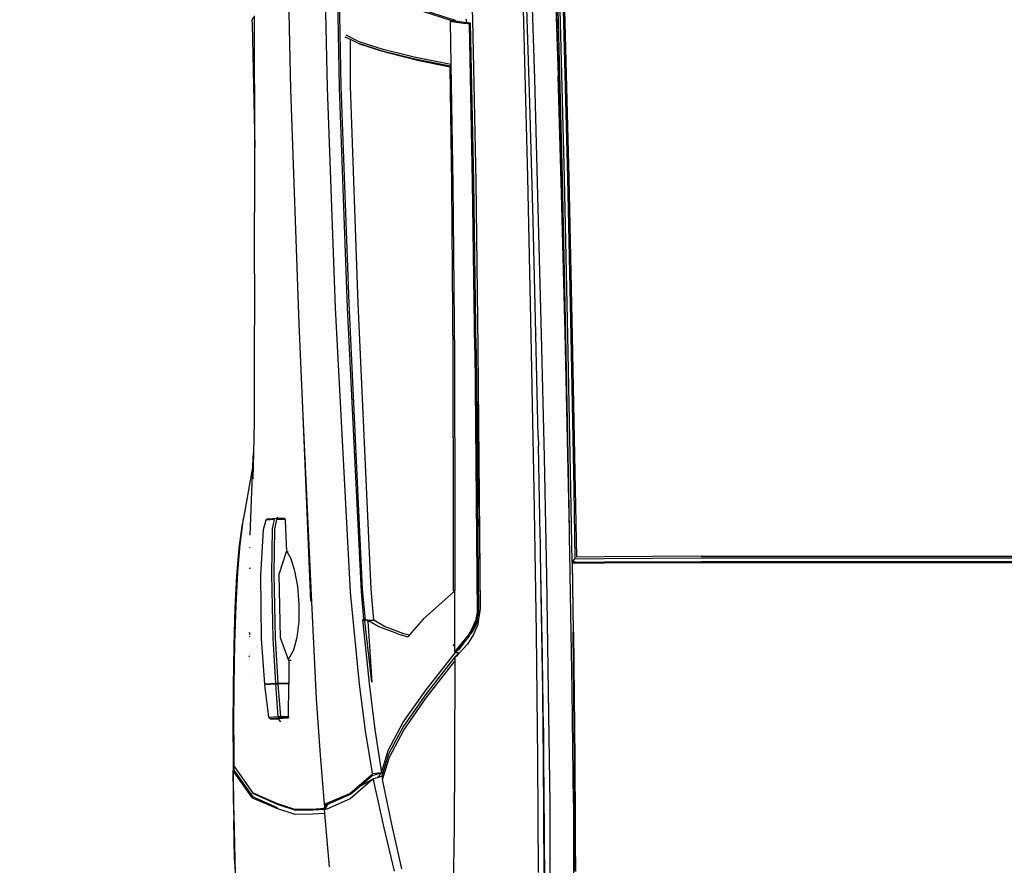
# Model space of a CAD drawing. Units: inches. Extents: x 1319 to 2030, y 219 to 1069.
# Tile 9 of 28: x 1417 to 1461, y 392 to 430. Entities that reach past the tile are written whole.
import ezdxf

# ---------------------------------------------------------------- set-up
doc = ezdxf.new("R2010")
doc.units = ezdxf.units.IN
doc.header["$MEASUREMENT"] = 0
doc.layers.get('0').update_dxf_attribs({"color": 12})
doc.layers.add('A-ANNO-DIMS', color=2, linetype='Continuous', lineweight=18)
doc.layers.add('C-PRKG-VEHC', color=8, linetype='Continuous', lineweight=13)
doc.layers.add('Edges', color=250, linetype='Continuous')
doc.styles.get("Standard").update_dxf_attribs({"font": 'arial.ttf'})
doc.dimstyles.get("Standard").update_dxf_attribs({"dimtxt": 7, "dimasz": 0.18, "dimexe": 0.18, "dimexo": 0.0625, "dimgap": 0.09, "dimtad": 0, "dimtih": 1, "dimtoh": 1, "dimzin": 0, "dimdsep": 46, "dimlunit": 3, "dimtxsty": 'Standard', "dimcen": 0.09, "dimadec": 0, "dimazin": 0, "dimtfac": 1, "dimtofl": 0, "dimtmove": 0, "dimatfit": 3, "dimfxl": 1, "dimtolj": 1, "dimtzin": 0, "dimarcsym": 0})

# ---------------------------------------------------------------- blocks, each defined once
blk = doc.blocks.new('Nissan Qashqai pl')
at = {"layer": 'Edges'}
for p, q in [((10.4706, 11.5566), (10.4706, 12.2875)), ((10.4726, 11.5567), (10.4726, 12.2875)), ((10.4764, 11.5569), (10.4764, 12.2872)), ((10.4776, 11.5567), (10.4776, 12.2874)), ((10.4706, 11.5566), (10.4711, 11.4469)), ((10.4731, 11.4469), (10.4726, 11.5567)), ((10.4769, 11.4474), (10.4764, 11.5569)), ((10.4781, 11.4469), (10.4776, 11.5567)), ((10.4711, 11.4469), (10.4715, 11.416)), ((10.4735, 11.414), (10.4731, 11.4469)), ((10.4773, 11.4146), (10.4769, 11.4474)), ((10.4785, 11.4111), (10.4781, 11.4469)), ((10.3947, 11.4148), (10.2218, 11.4114)), ((10.4715, 11.416), (10.3947, 11.4148)), ((10.4773, 11.4146), (10.4773, 11.4107)), ((10.7933, 11.4143), (10.827, 11.4145)), ((10.0431, 11.4075), (9.8673, 11.4031)), ((9.8673, 11.4012), (10.043, 11.4055)), ((10.2215, 11.406), (10.0429, 11.4021)), ((10.2216, 11.4037), (10.0429, 11.3998)), ((10.043, 11.4055), (10.2218, 11.4094)), ((10.2218, 11.4114), (10.0431, 11.4075)), ((10.3564, 11.406), (10.2175, 11.4028)), ((10.3945, 11.4094), (10.2215, 11.406)), ((10.3947, 11.4071), (10.2216, 11.4037)), ((10.2218, 11.4094), (10.3947, 11.4128)), ((10.4416, 11.4077), (10.3564, 11.406)), ((10.4773, 11.4107), (10.3945, 11.4094)), ((10.3947, 11.4128), (10.4735, 11.414)), ((10.4416, 11.4078), (10.3947, 11.4071)), ((10.4519, 11.4079), (10.4416, 11.4077)), ((10.4519, 11.4079), (10.4416, 11.4078)), ((10.4416, 11.4077), (10.4416, 11.4078)), ((10.4524, 11.408), (10.4519, 11.4079)), ((10.4519, 11.4079), (10.4519, 11.4079)), ((10.4524, 11.4079), (10.4519, 11.4079)), ((10.4524, 11.4079), (10.4524, 11.408)), ((10.4533, 11.408), (10.4524, 11.408)), ((10.4533, 11.4079), (10.4524, 11.4079)), ((10.4638, 11.4081), (10.4533, 11.4079)), ((10.4638, 11.4081), (10.4533, 11.408)), ((10.4533, 11.4079), (10.4533, 11.408)), ((10.4914, 11.4087), (10.4638, 11.4081)), ((10.4773, 11.4107), (10.4735, 11.414)), ((10.4773, 11.4107), (10.5561, 11.4119)), ((10.4773, 11.4107), (10.4785, 11.4111)), ((10.5563, 11.4123), (10.4785, 11.4111)), ((10.6223, 11.4109), (10.4914, 11.4087)), ((10.6996, 11.4134), (10.5561, 11.4119)), ((10.5563, 11.4123), (10.6999, 11.4138)), ((10.7493, 11.4125), (10.6223, 11.4109)), ((10.7722, 11.4138), (10.6996, 11.4134)), ((10.6999, 11.4138), (10.7722, 11.4142)), ((10.7493, 11.4125), (11.0294, 11.4126)), ((10.7722, 11.4142), (10.7889, 11.4143)), ((10.7722, 11.4142), (10.7722, 11.4138)), ((10.7889, 11.4139), (10.7722, 11.4138)), ((10.7889, 11.4139), (10.7889, 11.4143)), ((10.7889, 11.4143), (10.7923, 11.4143)), ((10.7923, 11.4139), (10.7889, 11.4139)), ((10.7923, 11.4139), (10.7923, 11.4143)), ((10.7923, 11.4143), (10.7933, 11.4143)), ((10.7933, 11.4139), (10.7923, 11.4139)), ((10.7933, 11.4139), (10.7933, 11.4143)), ((10.8267, 11.4141), (10.7933, 11.4139)), ((9.6472, 11.3861), (9.9278, 11.3949)), ((9.8673, 11.4031), (9.701, 11.3983)), ((9.7011, 11.3963), (9.8673, 11.4012)), ((9.8673, 11.3977), (9.7014, 11.3929)), ((9.8673, 11.3954), (9.7014, 11.3906)), ((9.8565, 11.3931), (9.9794, 11.3967)), ((10.0429, 11.4021), (9.8673, 11.3977)), ((10.0429, 11.3998), (9.8673, 11.3954)), ((10.0747, 11.3991), (9.9278, 11.3949)), ((9.9794, 11.3967), (10.0965, 11.3998)), ((10.2043, 11.4025), (10.0747, 11.3991)), ((10.0965, 11.3998), (10.0998, 11.3999)), ((10.0998, 11.3999), (10.2043, 11.4025)), ((10.2175, 11.4028), (10.2043, 11.4025)), ((10.3586, 11.3791), (10.4931, 11.3817)), ((10.4931, 11.3817), (10.6237, 11.3839)), ((10.6237, 11.3839), (10.7502, 11.3855)), ((10.7502, 11.3855), (10.968, 11.3857)), ((9.9312, 11.3681), (10.0776, 11.3722)), ((10.0776, 11.3722), (10.2201, 11.3759)), ((10.2201, 11.3759), (10.3586, 11.3791)), ((10.3353, 11.3725), (10.2203, 11.3699)), ((10.3353, 11.3725), (10.346, 11.3727)), ((10.4477, 11.3747), (10.346, 11.3727)), ((10.5572, 11.3704), (10.3955, 11.368)), ((10.4537, 11.3749), (10.4477, 11.3747)), ((10.4537, 11.3749), (10.4538, 11.3749)), ((10.4681, 11.3752), (10.4538, 11.3749)), ((10.4676, 11.3751), (10.4538, 11.3749)), ((10.5576, 11.3766), (10.4676, 11.3751)), ((10.5566, 11.3765), (10.4676, 11.3751)), ((10.4676, 11.3751), (10.4676, 11.3751)), ((10.5866, 11.3772), (10.4681, 11.3752)), ((10.5566, 11.3765), (10.7, 11.378)), ((10.7004, 11.372), (10.5572, 11.3704)), ((10.6649, 11.3783), (10.5576, 11.3766)), ((10.6649, 11.3783), (10.5866, 11.3772)), ((10.6908, 11.3785), (10.6649, 11.3783)), ((10.6649, 11.3783), (10.6772, 11.3784)), ((10.6966, 11.3787), (10.6772, 11.3784)), ((10.6772, 11.3784), (10.6908, 11.3785)), ((10.6991, 11.3786), (10.6908, 11.3785)), ((10.7144, 11.3788), (10.6966, 11.3787)), ((10.6999, 11.3786), (10.6991, 11.3786)), ((10.6999, 11.3786), (10.7808, 11.3793)), ((10.7144, 11.3788), (10.6999, 11.3786)), ((10.7, 11.378), (10.8279, 11.3787)), ((10.8279, 11.3727), (10.7004, 11.372)), ((10.7239, 11.3789), (10.7144, 11.3788)), ((10.7248, 11.3789), (10.7239, 11.3789)), ((10.7808, 11.3793), (10.7248, 11.3789)), ((10.7808, 11.3793), (10.8711, 11.3796)), ((9.9583, 11.363), (9.651, 11.3536)), ((9.6514, 11.3592), (9.9312, 11.3681)), ((10.0423, 11.3607), (9.8673, 11.3563)), ((10.091, 11.3666), (9.9583, 11.363)), ((10.2211, 11.3646), (10.0423, 11.3607)), ((10.2191, 11.3699), (10.091, 11.3666)), ((10.2202, 11.3699), (10.2191, 11.3699)), ((10.2202, 11.3699), (10.2203, 11.3699)), ((10.3955, 11.368), (10.2211, 11.3646)), ((9.8673, 11.3563), (9.7029, 11.3516)), ((10.0472, 11.3018), (10.2357, 11.3043)), ((10.2357, 11.3043), (10.53, 11.3068)), ((10.2367, 11.3022), (10.5351, 11.305)), ((10.2369, 11.3008), (10.5348, 11.3036)), ((10.4153, 11.3058), (10.2954, 11.3046)), ((10.4153, 11.3058), (10.4174, 11.3058)), ((10.4174, 11.3058), (10.4181, 11.3058)), ((10.4181, 11.3058), (10.4182, 11.3058)), ((10.4182, 11.3058), (10.53, 11.3068)), ((10.53, 11.3068), (10.5301, 11.3068)), ((10.5301, 11.3068), (10.5323, 11.3065)), ((10.5323, 11.3065), (10.5419, 11.3051)), ((10.5422, 11.3021), (10.5348, 11.3036)), ((10.5424, 11.3035), (10.5351, 11.305)), ((10.5366, 11.3048), (10.536, 11.305)), ((10.5379, 11.3052), (10.5381, 11.305)), ((10.5419, 11.3051), (10.5463, 11.3031)), ((10.5419, 11.3051), (10.5479, 11.3042)), ((10.5472, 11.3014), (10.5424, 11.3035)), ((10.5463, 11.3031), (10.5551, 11.2984)), ((10.5479, 11.3042), (10.5589, 11.2991)), ((9.696, 11.2932), (9.8644, 11.2982)), ((9.8644, 11.2982), (10.0472, 11.3018)), ((9.8678, 11.2935), (9.8677, 11.291)), ((9.8681, 11.2959), (9.8678, 11.2935)), ((10.0476, 11.2996), (9.8681, 11.2959)), ((9.8681, 11.2959), (9.869, 11.2946)), ((9.8689, 11.2927), (9.8686, 11.2879)), ((9.869, 11.2946), (9.8689, 11.2927)), ((10.0477, 11.2982), (9.869, 11.2946)), ((10.2367, 11.3022), (10.0476, 11.2996)), ((10.2369, 11.3008), (10.0477, 11.2982)), ((10.5522, 11.2977), (10.5422, 11.3021)), ((10.5546, 11.2982), (10.5472, 11.3014)), ((10.5598, 11.2935), (10.5522, 11.2977)), ((10.5583, 11.296), (10.5546, 11.2982)), ((10.5551, 11.2984), (10.5583, 11.296)), ((10.5612, 11.2944), (10.5583, 11.296)), ((10.5589, 11.2991), (10.57, 11.2925)), ((10.5764, 11.28), (10.5598, 11.2935)), ((10.5683, 11.2885), (10.5612, 11.2944)), ((10.57, 11.2925), (10.5811, 11.2822)), ((9.8637, 11.291), (9.8643, 11.291)), ((9.8643, 11.291), (9.8677, 11.291)), ((9.8675, 11.2887), (9.8655, 11.2754)), ((9.8686, 11.2879), (9.8665, 11.2747)), ((9.8677, 11.291), (9.8675, 11.2887)), ((10.5683, 11.2885), (10.573, 11.285)), ((10.575, 11.2829), (10.5683, 11.2885)), ((10.573, 11.285), (10.5769, 11.2818)), ((10.5776, 11.2808), (10.575, 11.2829)), ((10.5796, 11.2824), (10.5796, 11.2787)), ((10.5811, 11.2822), (10.5821, 11.2808)), ((10.5811, 11.2822), (10.5834, 11.28)), ((10.5821, 11.2808), (10.5834, 11.2793)), ((9.8652, 11.2788), (9.8516, 11.2363)), ((9.8652, 11.2738), (9.8516, 11.2313)), ((9.8652, 11.2738), (9.8652, 11.2788)), ((9.8655, 11.2754), (9.8652, 11.2738)), ((9.8652, 11.2735), (9.8665, 11.2747)), ((9.8652, 11.2738), (9.8652, 11.2738)), ((9.8652, 11.2738), (9.8652, 11.2735)), ((9.8652, 11.2735), (9.8664, 11.2728)), ((9.8665, 11.2747), (9.8664, 11.2728)), ((9.8664, 11.2728), (9.9149, 11.2736)), ((9.9149, 11.2736), (9.9066, 11.2322)), ((9.9169, 11.2728), (9.9086, 11.2313)), ((9.9177, 11.2728), (9.9106, 11.2373)), ((9.9149, 11.2736), (10.0505, 11.276)), ((9.9177, 11.2728), (9.9169, 11.2728)), ((10.0501, 11.2747), (9.9177, 11.2728)), ((10.2453, 11.2762), (10.0501, 11.2747)), ((10.0505, 11.276), (10.2453, 11.2777)), ((10.2453, 11.2777), (10.4289, 11.2783)), ((10.4292, 11.2767), (10.2453, 11.2762)), ((10.4289, 11.2783), (10.5092, 11.2783)), ((10.5099, 11.2768), (10.4292, 11.2767)), ((10.5099, 11.2768), (10.5092, 11.2783)), ((10.5092, 11.2783), (10.5094, 11.2783)), ((10.5094, 11.2783), (10.51, 11.2776)), ((10.5783, 11.2783), (10.5094, 11.2783)), ((10.51, 11.2776), (10.5099, 11.2768)), ((10.51, 11.2776), (10.5419, 11.2423)), ((10.5705, 11.2771), (10.5709, 11.2767)), ((10.5709, 11.2767), (10.5719, 11.2759)), ((10.5783, 11.2783), (10.5764, 11.28)), ((10.5796, 11.2787), (10.5776, 11.2808)), ((10.5776, 11.2808), (10.5783, 11.2783)), ((10.5796, 11.2787), (10.5783, 11.2783)), ((10.6215, 11.2456), (10.5796, 11.2787)), ((10.5825, 11.2806), (10.5834, 11.2793)), ((10.5834, 11.28), (10.5851, 11.2783)), ((10.5834, 11.2793), (10.5835, 11.2793)), ((10.5835, 11.2793), (10.584, 11.2787)), ((10.584, 11.2789), (10.584, 11.2793)), ((10.584, 11.2787), (10.584, 11.2789)), ((10.584, 11.2787), (10.6261, 11.2458)), ((10.584, 11.2787), (10.5851, 11.2783)), ((10.5843, 11.2787), (10.584, 11.2787)), ((10.5847, 11.2787), (10.5843, 11.2787)), ((10.5851, 11.2783), (10.5892, 11.2783)), ((10.6306, 11.2459), (10.5892, 11.2783)), ((10.5892, 11.2783), (10.6988, 11.2779)), ((10.6988, 11.2779), (10.7769, 11.2774)), ((10.7769, 11.2774), (10.858, 11.2759)), ((9.9106, 11.2373), (9.9018, 11.2021)), ((10.5419, 11.2423), (10.56, 11.2265)), ((10.6583, 11.2197), (10.6215, 11.2456)), ((10.6261, 11.2458), (10.6627, 11.22)), ((10.6671, 11.2203), (10.6306, 11.2459)), ((9.9066, 11.2322), (9.8978, 11.197)), ((9.9086, 11.2313), (9.8998, 11.196)), ((10.56, 11.2265), (10.5584, 11.2206)), ((10.56, 11.2265), (10.5617, 11.2251)), ((10.5584, 11.2206), (10.5502, 11.1986)), ((10.5584, 11.2136), (10.5617, 11.2251)), ((10.69, 11.2028), (10.6583, 11.2197)), ((10.6627, 11.22), (10.6943, 11.2032)), ((10.6976, 11.2041), (10.6671, 11.2203)), ((10.8239, 11.2181), (10.7754, 11.2071)), ((10.5584, 11.2136), (10.5502, 11.1916)), ((10.6943, 11.2032), (10.7155, 11.1969)), ((10.7228, 11.1965), (10.6976, 11.2041)), ((10.7754, 11.2071), (10.7228, 11.1965)), ((10.8264, 11.21), (10.7776, 11.1982)), ((9.8978, 11.197), (9.8891, 11.1701)), ((9.8911, 11.1693), (9.8998, 11.196)), ((9.9018, 11.2021), (9.8931, 11.1752)), ((10.5502, 11.1986), (10.543, 11.1865)), ((10.6664, 11.1875), (10.7155, 11.1952)), ((10.7155, 11.1952), (10.69, 11.2028)), ((10.7155, 11.1957), (10.7155, 11.1969)), ((10.7155, 11.1969), (10.7192, 11.1957)), ((10.7209, 11.1902), (10.7155, 11.1957)), ((10.7155, 11.1952), (10.7155, 11.1957)), ((10.7186, 11.1848), (10.7155, 11.1952)), ((10.7155, 11.1952), (10.7165, 11.1851)), ((10.7192, 11.1957), (10.7228, 11.1965)), ((10.7192, 11.1957), (10.7209, 11.1902)), ((10.7776, 11.1982), (10.7247, 11.1867)), ((10.5079, 11.1835), (10.1849, 11.1687)), ((10.543, 11.1865), (10.5079, 11.1835)), ((10.5502, 11.1916), (10.543, 11.1795)), ((10.543, 11.1795), (10.543, 11.1865)), ((10.5439, 11.1796), (10.613, 11.1841)), ((10.5458, 11.1742), (10.6144, 11.1813)), ((10.613, 11.1841), (10.547, 11.1767)), ((10.6144, 11.1813), (10.6664, 11.1875)), ((10.7137, 11.1846), (10.6678, 11.177)), ((10.7165, 11.1851), (10.7137, 11.1846)), ((10.7177, 11.1838), (10.7165, 11.1851)), ((10.7387, 11.1593), (10.7177, 11.1838)), ((10.7312, 11.1701), (10.7186, 11.1848)), ((10.7209, 11.1902), (10.7221, 11.1861)), ((10.7221, 11.1861), (10.7222, 11.1859)), ((10.7222, 11.186), (10.7221, 11.1861)), ((10.7247, 11.1867), (10.7222, 11.186)), ((10.7222, 11.186), (10.7222, 11.1859)), ((10.7222, 11.1859), (10.7232, 11.1848)), ((10.7222, 11.1859), (10.7224, 11.1855)), ((10.7224, 11.1855), (10.7312, 11.1701)), ((10.7232, 11.1848), (10.7228, 11.1859)), ((10.7232, 11.1848), (10.7449, 11.1598)), ((10.7257, 11.1853), (10.7256, 11.1854)), ((9.8891, 11.1701), (9.8818, 11.1551)), ((9.8931, 11.1751), (9.8911, 11.1693)), ((9.8931, 11.1751), (9.8931, 11.1752)), ((10.5079, 11.1739), (10.1849, 11.1585)), ((10.1894, 11.1563), (10.5109, 11.1721)), ((10.543, 11.1771), (10.5079, 11.1739)), ((10.5109, 11.1721), (10.5417, 11.1748)), ((10.6152, 11.1702), (10.5113, 11.1603)), ((10.543, 11.1771), (10.5417, 11.1748)), ((10.5417, 11.1748), (10.5427, 11.1739)), ((10.5436, 11.1754), (10.5427, 11.1739)), ((10.5427, 11.1739), (10.5458, 11.1742)), ((10.5439, 11.1796), (10.543, 11.1795)), ((10.543, 11.1795), (10.543, 11.1771)), ((10.544, 11.1763), (10.543, 11.1771)), ((10.544, 11.1763), (10.5436, 11.1754)), ((10.547, 11.1767), (10.544, 11.1763)), ((10.6678, 11.177), (10.6152, 11.1702)), ((10.7397, 11.1602), (10.7312, 11.1701)), ((9.8867, 11.16), (9.8838, 11.1541)), ((9.8911, 11.1691), (9.8867, 11.16)), ((9.9393, 11.1602), (9.8867, 11.16)), ((9.8911, 11.1693), (9.8911, 11.1691)), ((10.1849, 11.1687), (9.9393, 11.1602)), ((10.1849, 11.1585), (9.9393, 11.1497)), ((10.5113, 11.1603), (10.19, 11.1433)), ((10.7501, 11.1327), (10.7387, 11.1593)), ((10.7507, 11.1344), (10.7397, 11.1602)), ((10.7449, 11.1598), (10.7563, 11.1333)), ((9.8101, 11.1449), (9.9411, 11.1475)), ((9.9393, 11.1497), (9.8119, 11.1472)), ((9.9411, 11.1475), (10.1894, 11.1563)), ((10.19, 11.1433), (9.9414, 11.1341)), ((10.8218, 11.1365), (10.7615, 11.1311)), ((9.9414, 11.1341), (9.8143, 11.1312)), ((10.6318, 11.1213), (10.6955, 11.1257)), ((10.6955, 11.1257), (10.7509, 11.1302)), ((10.7507, 11.1309), (10.7501, 11.1327)), ((10.7511, 11.1335), (10.7507, 11.1344)), ((10.7507, 11.1344), (10.7524, 11.1335)), ((10.751, 11.131), (10.7507, 11.1309)), ((10.7509, 11.1302), (10.7507, 11.1309)), ((10.7522, 11.1311), (10.7509, 11.1302)), ((10.7516, 11.131), (10.7509, 11.1302)), ((10.7519, 11.1314), (10.7511, 11.1335)), ((10.7519, 11.1314), (10.7516, 11.131)), ((10.7522, 11.1311), (10.7516, 11.131)), ((10.7526, 11.1318), (10.7519, 11.1314)), ((10.7553, 11.1307), (10.7522, 11.1311)), ((10.7524, 11.1335), (10.7526, 11.1318)), ((10.7524, 11.1335), (10.7556, 11.1319)), ((10.7532, 11.1321), (10.7526, 11.1318)), ((10.7526, 11.1318), (10.7526, 11.1314)), ((10.7556, 11.1319), (10.7532, 11.1321)), ((10.7563, 11.1169), (10.7553, 11.1307)), ((10.7556, 11.1319), (10.7561, 11.1317)), ((10.7563, 11.1319), (10.7561, 11.1319)), ((10.7563, 11.1315), (10.7561, 11.1317)), ((10.7561, 11.1317), (10.7563, 11.1317)), ((10.7563, 11.1333), (10.7569, 11.1317)), ((10.7563, 11.1317), (10.7563, 11.1319)), ((10.7563, 11.1317), (10.7569, 11.1317)), ((10.7569, 11.1316), (10.7563, 11.1317)), ((10.7563, 11.1315), (10.7563, 11.1317)), ((10.7572, 11.1178), (10.7563, 11.1315)), ((10.7573, 11.1307), (10.7563, 11.1315)), ((10.7569, 11.1317), (10.7569, 11.1316)), ((10.7569, 11.1316), (10.7573, 11.1307)), ((10.7604, 11.131), (10.7573, 11.1307)), ((10.7615, 11.1311), (10.7604, 11.131)), ((10.7615, 11.1311), (10.7623, 11.1173)), ((10.312, 11.1064), (10.5147, 11.1156)), ((10.312, 11.1064), (10.5214, 11.1149)), ((10.5147, 11.1156), (10.6318, 11.1213)), ((10.7565, 11.0969), (10.7563, 11.1169)), ((10.7575, 11.0979), (10.7572, 11.1178)), ((10.7623, 11.1173), (10.7626, 11.0974)), ((10.2081, 11.1017), (10.312, 11.1064)), ((9.8024, 11.0892), (9.9426, 11.0923)), ((9.9426, 11.0923), (10.2081, 11.1017)), ((10.4653, 11.0881), (10.4732, 11.0925)), ((10.4732, 11.0925), (10.4871, 11.0967)), ((10.4871, 11.0967), (10.5048, 11.1002)), ((10.5048, 11.1002), (10.5246, 11.1019)), ((10.5246, 11.1019), (10.5445, 11.1017)), ((10.5445, 11.1017), (10.5625, 11.0996)), ((10.5625, 11.0996), (10.5769, 11.0957)), ((10.5769, 11.0957), (10.5863, 11.0904)), ((10.5885, 11.0931), (10.5885, 11.0904)), ((10.7497, 11.0763), (10.7565, 11.0969)), ((10.7507, 11.0773), (10.7575, 11.0979)), ((10.7626, 11.0974), (10.7559, 11.0767)), ((10.4274, 11.0767), (10.4275, 11.0856)), ((10.4275, 11.0856), (10.4293, 11.0863)), ((10.4293, 11.0863), (10.4291, 11.0765)), ((10.4293, 11.0863), (10.4398, 11.0868)), ((10.4398, 11.0868), (10.4653, 11.0878)), ((10.4653, 11.0881), (10.4652, 11.0897)), ((10.4653, 11.0877), (10.4653, 11.0881)), ((10.4653, 11.0878), (10.4653, 11.0881)), ((10.4653, 11.0881), (10.4653, 11.0881)), ((10.4653, 11.0877), (10.4653, 11.0878)), ((10.4908, 11.0793), (10.4653, 11.0877)), ((10.563, 11.0809), (10.4908, 11.0793)), ((10.5867, 11.0897), (10.563, 11.0809)), ((10.5863, 11.0904), (10.5867, 11.0897)), ((10.5885, 11.0904), (10.5867, 11.0897)), ((10.5885, 11.0904), (10.6141, 11.0905)), ((10.6141, 11.0905), (10.615, 11.0905)), ((10.6142, 11.0782), (10.6141, 11.0905)), ((10.6517, 11.0902), (10.615, 11.0905)), ((10.615, 11.0905), (10.6151, 11.0782)), ((10.6151, 11.078), (10.6518, 11.0808)), ((10.6518, 11.0808), (10.6517, 11.0902)), ((10.6517, 11.0902), (10.6535, 11.0895)), ((10.6518, 11.0784), (10.6518, 11.0808)), ((10.6518, 11.0808), (10.6536, 11.0803)), ((10.6535, 11.0895), (10.6543, 11.0786)), ((10.6535, 11.0895), (10.6536, 11.0803)), ((10.6578, 11.0814), (10.6543, 11.0786)), ((10.4263, 11.0777), (10.4274, 11.0767)), ((10.4274, 11.0762), (10.4274, 11.0767)), ((10.4282, 11.0666), (10.4274, 11.0762)), ((10.4291, 11.0765), (10.4398, 11.0741)), ((10.4398, 11.0718), (10.4291, 11.0741)), ((10.4291, 11.0741), (10.4299, 11.0644)), ((10.4398, 11.0741), (10.4909, 11.0734)), ((10.4909, 11.0711), (10.4398, 11.0718)), ((10.4909, 11.0734), (10.563, 11.075)), ((10.5631, 11.0727), (10.4909, 11.0711)), ((10.563, 11.075), (10.6142, 11.0779)), ((10.6142, 11.0756), (10.5631, 11.0727)), ((10.6142, 11.0779), (10.6142, 11.0782)), ((10.6142, 11.0765), (10.6142, 11.0779)), ((10.615, 11.0765), (10.6142, 11.0765)), ((10.6142, 11.0756), (10.6142, 11.0765)), ((10.615, 11.0639), (10.6142, 11.0756)), ((10.6151, 11.0765), (10.615, 11.0765)), ((10.615, 11.0765), (10.6151, 11.0639)), ((10.6518, 11.0784), (10.6151, 11.0756)), ((10.6151, 11.0782), (10.6151, 11.078)), ((10.6151, 11.078), (10.6151, 11.0765)), ((10.6151, 11.0765), (10.6151, 11.0756)), ((10.6151, 11.0756), (10.616, 11.0629)), ((10.6536, 11.0803), (10.6518, 11.0784)), ((10.6526, 11.0674), (10.6518, 11.0784)), ((10.6526, 11.0674), (10.6543, 11.0693)), ((10.6536, 11.0803), (10.6537, 11.0783)), ((10.6543, 11.0786), (10.6537, 11.0783)), ((10.6537, 11.0783), (10.6543, 11.0693)), ((10.6543, 11.0693), (10.6543, 11.0786)), ((10.7385, 11.051), (10.7497, 11.0763)), ((10.7396, 11.0519), (10.7507, 11.0773)), ((10.7549, 11.0776), (10.743, 11.0503)), ((10.7559, 11.0767), (10.7448, 11.0511)), ((10.4282, 11.0666), (10.4299, 11.0644)), ((10.4299, 11.0644), (10.4406, 11.0612)), ((10.4406, 11.0612), (10.4919, 11.0584)), ((10.4919, 11.0584), (10.564, 11.0591)), ((10.564, 11.0591), (10.6151, 11.0628)), ((10.6151, 11.0639), (10.615, 11.0639)), ((10.6151, 11.0628), (10.615, 11.0639)), ((10.6151, 11.0639), (10.6151, 11.0628)), ((10.616, 11.0629), (10.6526, 11.0674)), ((9.8643, 11.0514), (9.8598, 11.0514)), ((9.8614, 11.0504), (9.8647, 11.0485)), ((10.0085, 11.0519), (9.8643, 11.0514)), ((9.8647, 11.0485), (9.869, 11.0488)), ((9.869, 11.0488), (10.0085, 11.0519)), ((10.0124, 11.0519), (10.0085, 11.0519)), ((10.1513, 11.0517), (10.0124, 11.0519)), ((10.1513, 11.0517), (10.2677, 11.0512)), ((10.2677, 11.0512), (10.3189, 11.0511)), ((10.3189, 11.0511), (10.3537, 11.0503)), ((10.3537, 11.0503), (10.3832, 11.0496)), ((10.3679, 11.0497), (10.3537, 11.0503)), ((10.3679, 11.0497), (10.4275, 11.0391)), ((10.4468, 11.0466), (10.3679, 11.0497)), ((10.7087, 11.0289), (10.7363, 11.0483)), ((10.7424, 11.0499), (10.7125, 11.0285)), ((10.7429, 11.0485), (10.7148, 11.0284)), ((10.7363, 11.0483), (10.7376, 11.0492)), ((10.7387, 11.0502), (10.7376, 11.0492)), ((10.7376, 11.0492), (10.7378, 11.0495)), ((10.7378, 11.0495), (10.7385, 11.051)), ((10.7378, 11.0495), (10.7379, 11.0496)), ((10.7387, 11.0502), (10.7396, 11.0519)), ((10.7424, 11.0499), (10.743, 11.0503)), ((10.7429, 11.0488), (10.7432, 11.0488)), ((10.7432, 11.0488), (10.7429, 11.0485)), ((10.744, 11.0494), (10.7432, 11.0488)), ((10.7448, 11.0511), (10.744, 11.0494)), ((10.4275, 11.0391), (10.4304, 11.0385)), ((10.4304, 11.0385), (10.4339, 11.0381)), ((10.4345, 11.0379), (10.4339, 11.0381)), ((10.4339, 11.0381), (10.4573, 11.0349)), ((10.4613, 11.0343), (10.4345, 11.0379)), ((10.4502, 11.0466), (10.4503, 11.0465)), ((10.4613, 11.0464), (10.4603, 11.0465)), ((10.4838, 11.0465), (10.4852, 11.046)), ((10.5565, 11.0456), (10.5591, 11.0464)), ((10.5615, 11.0464), (10.5617, 11.0457)), ((10.583, 11.0457), (10.5835, 11.0461)), ((10.5836, 11.0461), (10.5832, 11.0457)), ((10.5847, 11.0461), (10.5841, 11.0457)), ((10.5873, 11.0461), (10.5873, 11.0461)), ((10.6087, 11.0458), (10.6087, 11.0458)), ((10.4573, 11.0349), (10.4889, 11.0323)), ((10.4926, 11.0317), (10.4613, 11.0343)), ((10.4889, 11.0323), (10.526, 11.0304)), ((10.5294, 11.0298), (10.4926, 11.0317)), ((10.526, 11.0304), (10.569, 11.0291)), ((10.5719, 11.0285), (10.5294, 11.0298)), ((10.569, 11.0291), (10.5919, 11.0287)), ((10.6176, 11.0277), (10.5719, 11.0285)), ((10.5919, 11.0287), (10.5936, 11.0286)), ((10.5936, 11.0286), (10.6151, 11.0283)), ((10.6151, 11.0283), (10.6644, 11.028)), ((10.6651, 11.0274), (10.6176, 11.0277)), ((10.6644, 11.028), (10.7078, 11.0282)), ((10.677, 11.0275), (10.6651, 11.0274)), ((10.7082, 11.0285), (10.6729, 11.0284)), ((10.68, 11.0274), (10.677, 11.0275)), ((10.6809, 11.0274), (10.68, 11.0274)), ((10.6809, 11.0274), (10.7128, 11.0275)), ((10.7078, 11.0282), (10.7083, 11.0285)), ((10.7082, 11.0285), (10.7078, 11.0282)), ((10.7085, 11.0289), (10.7082, 11.0285)), ((10.7083, 11.0285), (10.7082, 11.0285)), ((10.7083, 11.0285), (10.7087, 11.0289)), ((10.7125, 11.0285), (10.7083, 11.0285)), ((10.7146, 11.0286), (10.7125, 11.0285)), ((10.7125, 11.0285), (10.7139, 11.0278)), ((10.7134, 11.0275), (10.7128, 11.0275)), ((10.7625, 11.0281), (10.7134, 11.0275)), ((10.724, 11.0275), (10.7134, 11.0275)), ((10.7148, 11.0284), (10.7139, 11.0278)), ((10.7628, 11.0283), (10.7139, 11.0278)), ((10.724, 11.0275), (10.7685, 11.0281)), ((10.7628, 11.0281), (10.7625, 11.0281)), ((10.7628, 11.0283), (10.8131, 11.0292)), ((10.7628, 11.0281), (10.8131, 11.029)), ((10.7688, 11.0281), (10.7685, 11.0281)), ((10.8131, 11.029), (10.7688, 11.0281)), ((10.8131, 11.0292), (10.8644, 11.0306)), ((10.8132, 11.029), (10.8131, 11.029)), ((10.8132, 11.029), (10.8139, 11.029)), ((10.8142, 11.029), (10.8139, 11.029)), ((10.8142, 11.029), (10.8241, 11.0293)), ((10.8142, 11.029), (10.8142, 11.029))]:
    blk.add_line(p, q, dxfattribs=at)
blk = doc.blocks.new('car')
blk.add_blockref('Nissan Qashqai pl', (-9.7433, -11.9151))
blk = doc.blocks.new('carr')
blk.add_blockref('car', (0.5124, -0.007))
blk = doc.blocks.new('*D56')
at = {"layer": 'A-ANNO-DIMS', "color": 0, "lineweight": -2, "transparency": 16777216}
for p, q in [((1419.852, 531.201), (1393.865, 531.201)), ((1394.045, 531.021), (1394.045, 448.679)), ((1394.045, 358.918), (1394.045, 441.26)), ((1419.852, 358.738), (1393.865, 358.738))]:
    blk.add_line(p, q, dxfattribs=at)
at = {"layer": 'A-ANNO-DIMS', "color": 0, "transparency": 16777216}
for points in [[(1394.015, 531.021), (1394.075, 531.021), (1394.045, 531.201)], [(1394.015, 358.918), (1394.075, 358.918), (1394.045, 358.738)]]:
    blk.add_solid(points, dxfattribs=at)
at = {"layer": 'Defpoints', "color": 0, "transparency": 16777216}
for p in [(1419.914, 531.201), (1394.045, 358.738), (1419.914, 358.738)]:
    blk.add_point(p, dxfattribs=at)
at = {"layer": 'A-ANNO-DIMS', "color": 0, "transparency": 16777216, "insert": (1394.045, 444.969), "char_height": 7, "attachment_point": 5}
blk.add_mtext('\\A1;CAR 14\'-4 1/2"', dxfattribs=at)
blk = doc.blocks.new('*D65')
at = {"layer": 'A-ANNO-DIMS', "color": 0, "lineweight": -2, "transparency": 16777216}
for p, q in [((1648.280254, 472.227245), (1329.112754, 472.227245)), ((1329.292754, 472.047245), (1329.292754, 431.817245)), ((1329.292754, 384.407245), (1329.292754, 424.637245)), ((1648.280254, 384.227245), (1329.112754, 384.227245))]:
    blk.add_line(p, q, dxfattribs=at)
at = {"layer": 'A-ANNO-DIMS', "color": 0, "transparency": 16777216}
for points in [[(1329.262754, 472.047245), (1329.322754, 472.047245), (1329.292754, 472.227245)], [(1329.262754, 384.407245), (1329.322754, 384.407245), (1329.292754, 384.227245)]]:
    blk.add_solid(points, dxfattribs=at)
at = {"layer": 'Defpoints', "color": 0, "transparency": 16777216}
for p in [(1329.292754, 472.227245), (1648.342754, 472.227245), (1648.342754, 384.227245)]:
    blk.add_point(p, dxfattribs=at)
at = {"layer": 'A-ANNO-DIMS', "color": 0, "transparency": 16777216, "insert": (1329.292754, 428.227245), "char_height": 7, "attachment_point": 5}
blk.add_mtext('\\A1;7\'-4"', dxfattribs=at)

msp = doc.modelspace()

# ---------------------------------------------------------------- block references
at = {"layer": 'C-PRKG-VEHC', "xscale": 39.37007874015748, "yscale": 39.37007874015748, "zscale": 39.37007874015748, "rotation": 270}
msp.add_blockref('carr', (1462.179, 454.621), dxfattribs=at)

# ---------------------------------------------------------------- dimensions: what is measured, and where the dimension line sits
at = {"layer": 'A-ANNO-DIMS'}
dim = msp.add_linear_dim(base=(1394.045, 358.738), p1=(1419.914, 531.201), p2=(1419.914, 358.738), angle=270, text='CAR <>', dimstyle='Standard', override={"dimdec": 1, "dimlfac": 1, "dimrnd": 0, "dimzin": 1, "dimdsep": 46, "dimlunit": 4, "dimfrac": 2}, dxfattribs=at)
dim.commit()
dim.dimension.update_dxf_attribs({"geometry": '*D56', "text_midpoint": (1394.045, 444.969)})
dim = msp.add_linear_dim(base=(1329.293, 472.227), p1=(1648.343, 384.227), p2=(1648.343, 472.227), angle=90, dimstyle='Standard', override={"dimdec": 1, "dimlfac": 1, "dimrnd": 0, "dimzin": 1, "dimdsep": 46, "dimlunit": 4, "dimfrac": 2}, dxfattribs=at)
dim.commit()
dim.dimension.update_dxf_attribs({"geometry": '*D65', "text_midpoint": (1329.293, 428.227)})

doc.saveas('drawing.dxf')
